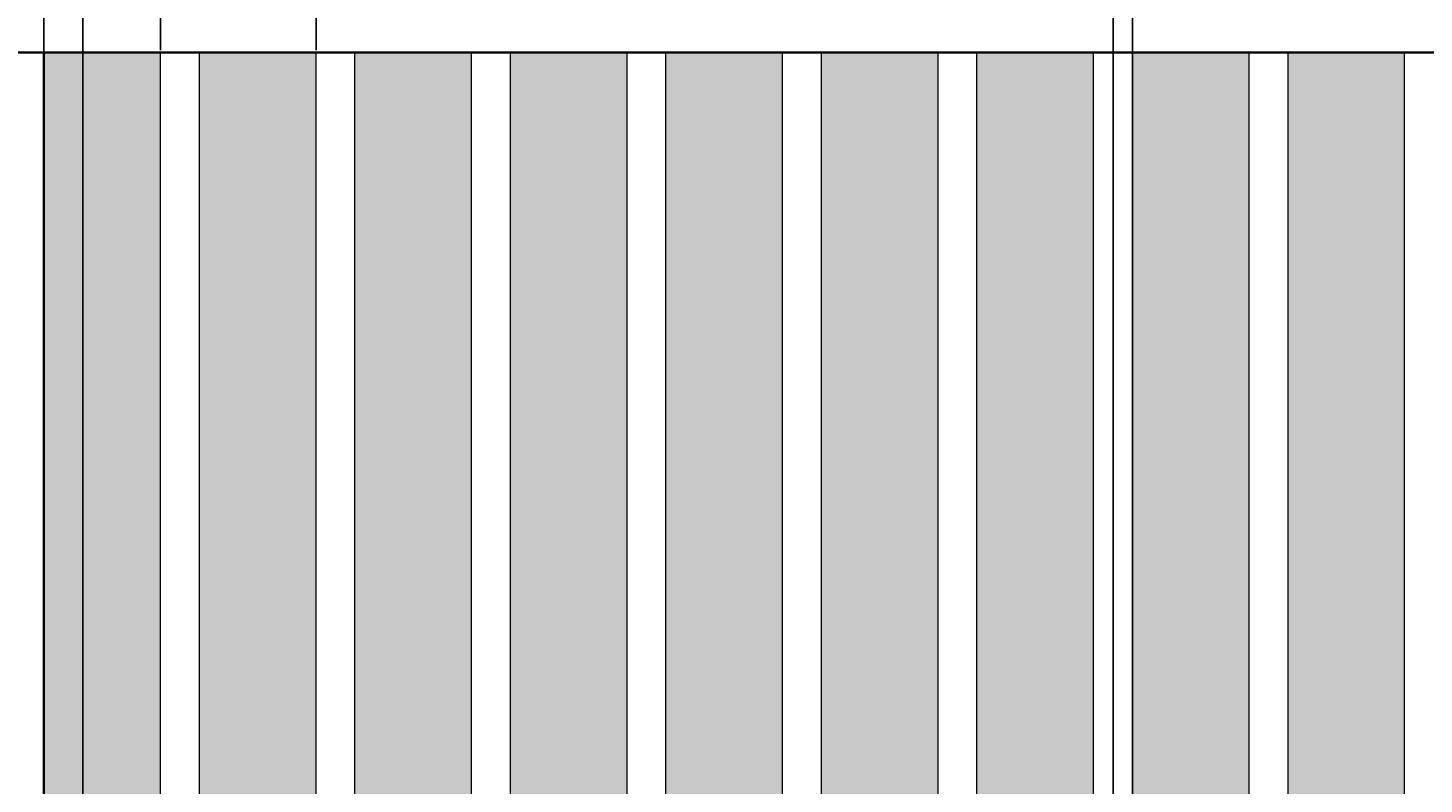
# Model space of a CAD drawing. Units: inches. Extents: x 4508 to 4723, y 847 to 1020.
# Tile 15 of 32: x 4550 to 4585, y 976 to 995. Entities that reach past the tile are written whole.
import ezdxf

# ---------------------------------------------------------------- set-up
doc = ezdxf.new("R2010")
doc.units = ezdxf.units.IN
for name, color, linetype, lineweight in [('A-ANNO-DIMS', 2, 'Continuous', 18), ('A-WALL', 7, 'Continuous', 35), ('A-WALL-FINS', 30, 'Continuous', 18), ('A-WALL-PATT', 254, 'Continuous', 13)]:
    doc.layers.add(name, color=color, linetype=linetype, lineweight=lineweight)
doc.styles.get("Standard").update_dxf_attribs({"font": 'arial.ttf'})
doc.dimstyles.get("Standard").update_dxf_attribs({"dimtxt": 0.18, "dimasz": 0.18, "dimexe": 0.18, "dimexo": 0.0625, "dimgap": 0.09, "dimtad": 0, "dimtih": 1, "dimtoh": 1, "dimdec": 4, "dimzin": 0, "dimdsep": 46, "dimtxsty": 'Standard', "dimcen": 0.09, "dimadec": 0, "dimazin": 0, "dimtfac": 1, "dimtdec": 4, "dimtofl": 0, "dimtmove": 0, "dimatfit": 3, "dimfxl": 1, "dimtolj": 1, "dimtzin": 0, "dimarcsym": 0})

# ---------------------------------------------------------------- blocks, each defined once
blk = doc.blocks.new('*D4')
at = {"layer": 'A-ANNO-DIMS', "color": 0, "lineweight": -2, "transparency": 16777216}
for p, q in [((4540.994, 994.809), (4540.994, 1002.877)), ((4541.174, 1002.697), (4545.345, 1002.697)), ((4549.814, 1002.697), (4545.643, 1002.697)), ((4549.994, 994.809), (4549.994, 1002.877))]:
    blk.add_line(p, q, dxfattribs=at)
at = {"layer": 'A-ANNO-DIMS', "color": 0, "lineweight": 9, "transparency": 16777216}
for points in [[(4541.174, 1002.727), (4541.174, 1002.667), (4540.994, 1002.697)], [(4549.814, 1002.727), (4549.814, 1002.667), (4549.994, 1002.697)]]:
    blk.add_solid(points, dxfattribs=at)
at = {"layer": 'Defpoints', "color": 0, "lineweight": 9, "transparency": 16777216}
for p in [(4549.994, 1002.697), (4540.994, 994.747), (4549.994, 994.747)]:
    blk.add_point(p, dxfattribs=at)
at = {"layer": 'A-ANNO-DIMS', "color": 0, "transparency": 16777216, "insert": (4545.494, 1002.697), "char_height": 0.18, "attachment_point": 5}
blk.add_mtext('\\A1;9', dxfattribs=at)
blk = doc.blocks.new('*D5')
at = {"layer": 'A-ANNO-DIMS', "color": 0, "lineweight": -2, "transparency": 16777216}
for p, q in [((4549.994, 994.809), (4549.994, 1002.877)), ((4550.174, 1002.697), (4551.345, 1002.697)), ((4552.814, 1002.697), (4551.643, 1002.697)), ((4552.994, 994.809), (4552.994, 1002.877))]:
    blk.add_line(p, q, dxfattribs=at)
at = {"layer": 'A-ANNO-DIMS', "color": 0, "lineweight": 9, "transparency": 16777216}
for points in [[(4550.174, 1002.727), (4550.174, 1002.667), (4549.994, 1002.697)], [(4552.814, 1002.727), (4552.814, 1002.667), (4552.994, 1002.697)]]:
    blk.add_solid(points, dxfattribs=at)
at = {"layer": 'Defpoints', "color": 0, "lineweight": 9, "transparency": 16777216}
for p in [(4552.994, 1002.697), (4549.994, 994.747), (4552.994, 994.747)]:
    blk.add_point(p, dxfattribs=at)
at = {"layer": 'A-ANNO-DIMS', "color": 0, "transparency": 16777216, "insert": (4551.494, 1002.697), "char_height": 0.18, "attachment_point": 5}
blk.add_mtext('\\A1;3', dxfattribs=at)
blk = doc.blocks.new('*D6')
at = {"layer": 'A-ANNO-DIMS', "color": 0, "lineweight": -2, "transparency": 16777216}
for p, q in [((4552.994, 994.809), (4552.994, 1002.877)), ((4553.174, 1002.697), (4554.842, 1002.697)), ((4556.814, 1002.697), (4555.146, 1002.697)), ((4556.994, 994.809), (4556.994, 1002.877))]:
    blk.add_line(p, q, dxfattribs=at)
at = {"layer": 'A-ANNO-DIMS', "color": 0, "lineweight": 9, "transparency": 16777216}
for points in [[(4553.174, 1002.727), (4553.174, 1002.667), (4552.994, 1002.697)], [(4556.814, 1002.727), (4556.814, 1002.667), (4556.994, 1002.697)]]:
    blk.add_solid(points, dxfattribs=at)
at = {"layer": 'Defpoints', "color": 0, "lineweight": 9, "transparency": 16777216}
for p in [(4556.994, 1002.697), (4552.994, 994.747), (4556.994, 994.747)]:
    blk.add_point(p, dxfattribs=at)
at = {"layer": 'A-ANNO-DIMS', "color": 0, "transparency": 16777216, "insert": (4554.994, 1002.697), "char_height": 0.18, "attachment_point": 5}
blk.add_mtext('\\A1;4', dxfattribs=at)
blk = doc.blocks.new('*D26')
at = {"layer": 'A-ANNO-DIMS', "color": 0, "lineweight": -2, "transparency": 16777216}
for p, q in [((4549.994, 904.809), (4549.994, 1002.877)), ((4550.174, 1002.697), (4550.371, 1002.697)), ((4550.814, 1002.697), (4550.617, 1002.697)), ((4550.994, 903.809), (4550.994, 1002.877))]:
    blk.add_line(p, q, dxfattribs=at)
at = {"layer": 'A-ANNO-DIMS', "color": 0, "lineweight": 9, "transparency": 16777216}
for points in [[(4550.174, 1002.727), (4550.174, 1002.667), (4549.994, 1002.697)], [(4550.814, 1002.727), (4550.814, 1002.667), (4550.994, 1002.697)]]:
    blk.add_solid(points, dxfattribs=at)
at = {"layer": 'Defpoints', "color": 0, "lineweight": 9, "transparency": 16777216}
for p in [(4550.994, 1002.697), (4549.994, 904.747), (4550.994, 903.747)]:
    blk.add_point(p, dxfattribs=at)
at = {"layer": 'A-ANNO-DIMS', "color": 0, "transparency": 16777216, "insert": (4550.494, 1002.697), "char_height": 0.18, "attachment_point": 5}
blk.add_mtext('\\A1;1', dxfattribs=at)
blk = doc.blocks.new('*D27')
at = {"layer": 'A-ANNO-DIMS', "color": 0, "lineweight": -2, "transparency": 16777216}
for p, q in [((4550.994, 903.809), (4550.994, 1002.877)), ((4551.174, 1002.697), (4563.918, 1002.697)), ((4577.314, 1002.697), (4564.57, 1002.697)), ((4577.494, 903.809), (4577.494, 1002.877))]:
    blk.add_line(p, q, dxfattribs=at)
at = {"layer": 'A-ANNO-DIMS', "color": 0, "lineweight": 9, "transparency": 16777216}
for points in [[(4551.174, 1002.727), (4551.174, 1002.667), (4550.994, 1002.697)], [(4577.314, 1002.727), (4577.314, 1002.667), (4577.494, 1002.697)]]:
    blk.add_solid(points, dxfattribs=at)
at = {"layer": 'Defpoints', "color": 0, "lineweight": 9, "transparency": 16777216}
for p in [(4577.494, 1002.697), (4550.994, 903.747), (4577.494, 903.747)]:
    blk.add_point(p, dxfattribs=at)
at = {"layer": 'A-ANNO-DIMS', "color": 0, "transparency": 16777216, "insert": (4564.244, 1002.697), "char_height": 0.18, "attachment_point": 5}
blk.add_mtext('\\A1;26.5', dxfattribs=at)
blk = doc.blocks.new('*D28')
at = {"layer": 'A-ANNO-DIMS', "color": 0, "lineweight": -2, "transparency": 16777216}
for p, q in [((4577.314, 1002.697), (4577.134, 1002.697)), ((4577.494, 903.809), (4577.494, 1002.877)), ((4577.994, 903.809), (4577.994, 1002.877)), ((4578.174, 1002.697), (4578.354, 1002.697))]:
    blk.add_line(p, q, dxfattribs=at)
at = {"layer": 'A-ANNO-DIMS', "color": 0, "lineweight": 9, "transparency": 16777216}
for points in [[(4577.314, 1002.727), (4577.314, 1002.667), (4577.494, 1002.697)], [(4578.174, 1002.727), (4578.174, 1002.667), (4577.994, 1002.697)]]:
    blk.add_solid(points, dxfattribs=at)
at = {"layer": 'Defpoints', "color": 0, "lineweight": 9, "transparency": 16777216}
for p in [(4577.994, 1002.697), (4577.494, 903.747), (4577.994, 903.747)]:
    blk.add_point(p, dxfattribs=at)
at = {"layer": 'A-ANNO-DIMS', "color": 0, "transparency": 16777216, "insert": (4578.608, 1002.697), "char_height": 0.18, "attachment_point": 5}
blk.add_mtext('\\A1;0.5', dxfattribs=at)
blk = doc.blocks.new('*D29')
at = {"layer": 'A-ANNO-DIMS', "color": 0, "lineweight": -2, "transparency": 16777216}
for p, q in [((4577.994, 903.809), (4577.994, 1002.877)), ((4578.174, 1002.697), (4590.773, 1002.697)), ((4603.814, 1002.697), (4591.214, 1002.697)), ((4603.994, 903.809), (4603.994, 1002.877))]:
    blk.add_line(p, q, dxfattribs=at)
at = {"layer": 'A-ANNO-DIMS', "color": 0, "lineweight": 9, "transparency": 16777216}
for points in [[(4578.174, 1002.727), (4578.174, 1002.667), (4577.994, 1002.697)], [(4603.814, 1002.727), (4603.814, 1002.667), (4603.994, 1002.697)]]:
    blk.add_solid(points, dxfattribs=at)
at = {"layer": 'Defpoints', "color": 0, "lineweight": 9, "transparency": 16777216}
for p in [(4603.994, 1002.697), (4577.994, 903.747), (4603.994, 903.747)]:
    blk.add_point(p, dxfattribs=at)
at = {"layer": 'A-ANNO-DIMS', "color": 0, "transparency": 16777216, "insert": (4590.994, 1002.697), "char_height": 0.18, "attachment_point": 5}
blk.add_mtext('\\A1;26', dxfattribs=at)

msp = doc.modelspace()

# ---------------------------------------------------------------- hatches: boundary and pattern name
at = {"layer": 'A-WALL-PATT', "transparency": 33554681}
h = msp.add_hatch(color=256, dxfattribs=at)
h.dxf.hatch_style = 1
h.paths.add_polyline_path([(4552.9938, 994.7469), (4549.9938, 994.7469), (4549.9938, 904.7469), (4552.9938, 904.7469)])
h.paths.add_polyline_path([(4556.9938, 994.7469), (4553.9938, 994.7469), (4553.9938, 904.7469), (4556.9938, 904.7469)])
h.paths.add_polyline_path([(4560.9938, 994.7469), (4557.9938, 994.7469), (4557.9938, 904.7469), (4560.9938, 904.7469)])
h.paths.add_polyline_path([(4564.9938, 994.7469), (4561.9938, 994.7469), (4561.9938, 904.7469), (4564.9938, 904.7469)])
h.paths.add_polyline_path([(4568.9938, 994.7469), (4565.9938, 994.7469), (4565.9938, 904.7469), (4568.9938, 904.7469)])
h.paths.add_polyline_path([(4572.9938, 994.7469), (4569.9938, 994.7469), (4569.9938, 904.7469), (4572.9938, 904.7469)])
h.paths.add_polyline_path([(4576.9938, 994.7469), (4573.9938, 994.7469), (4573.9938, 904.7469), (4576.9938, 904.7469)])
h.paths.add_polyline_path([(4580.9938, 994.7469), (4577.9938, 994.7469), (4577.9938, 904.7469), (4580.9938, 904.7469)])
h.paths.add_polyline_path([(4584.9938, 994.7469), (4581.9938, 994.7469), (4581.9938, 904.7469), (4584.9938, 904.7469)])

# ---------------------------------------------------------------- linework, layer by layer
at = {"layer": 'A-WALL'}
for p, q in [((4540.9938, 994.7469), (4693.9938, 994.7469)), ((4549.9938, 874.7469), (4549.9938, 994.7469))]:
    msp.add_line(p, q, dxfattribs=at)
at = {"layer": 'A-WALL-FINS'}
for p, q in [((4552.9938, 904.7469), (4552.9938, 994.7469)), ((4553.9938, 904.7469), (4553.9938, 994.7469)), ((4556.9938, 904.7469), (4556.9938, 994.7469)), ((4557.9938, 904.7469), (4557.9938, 994.7469)), ((4560.9938, 904.7469), (4560.9938, 994.7469)), ((4561.9938, 904.7469), (4561.9938, 994.7469)), ((4564.9938, 904.7469), (4564.9938, 994.7469)), ((4565.9938, 904.7469), (4565.9938, 994.7469)), ((4568.9938, 904.7469), (4568.9938, 994.7469)), ((4569.9938, 904.7469), (4569.9938, 994.7469)), ((4572.9938, 904.7469), (4572.9938, 994.7469)), ((4573.9938, 904.7469), (4573.9938, 994.7469)), ((4576.9938, 904.7469), (4576.9938, 994.7469)), ((4577.9938, 904.7469), (4577.9938, 994.7469)), ((4580.9938, 904.7469), (4580.9938, 994.7469)), ((4581.9938, 904.7469), (4581.9938, 994.7469)), ((4584.9938, 904.7469), (4584.9938, 994.7469))]:
    msp.add_line(p, q, dxfattribs=at)

# ---------------------------------------------------------------- dimensions: what is measured, and where the dimension line sits
at = {"layer": 'A-ANNO-DIMS'}
for base, p1, p2, override, picture, middle in [((4549.9938, 1002.6969), (4540.9938, 994.7469), (4549.9938, 994.7469), {"dimdec": 0, "dimlfac": 1, "dimrnd": 0, "dimzin": 0, "dimdsep": 46, "dimlunit": 2}, '*D4', (4545.4938, 1002.6969)), ((4552.9938, 1002.6969), (4549.9938, 994.7469), (4552.9938, 994.7469), {"dimdec": 0, "dimlfac": 1, "dimrnd": 0, "dimzin": 0, "dimdsep": 46, "dimlunit": 2}, '*D5', (4551.4938, 1002.6969)), ((4550.9938, 1002.6969), (4549.9938, 904.7469), (4550.9938, 903.7469), {"dimdec": 0, "dimlfac": 1, "dimrnd": 0, "dimzin": 0, "dimdsep": 46, "dimlunit": 2}, '*D26', (4550.4938, 1002.6969)), ((4577.4938, 1002.6969), (4550.9938, 903.7469), (4577.4938, 903.7469), {"dimdec": 1, "dimlfac": 1, "dimrnd": 0, "dimzin": 0, "dimdsep": 46, "dimlunit": 2}, '*D27', (4564.2438, 1002.6969)), ((4556.9938, 1002.6969), (4552.9938, 994.7469), (4556.9938, 994.7469), {"dimdec": 0, "dimlfac": 1, "dimrnd": 0, "dimzin": 0, "dimdsep": 46, "dimlunit": 2}, '*D6', (4554.9938, 1002.6969)), ((4577.9938, 1002.6969), (4577.4938, 903.7469), (4577.9938, 903.7469), {"dimdec": 1, "dimlfac": 1, "dimrnd": 0, "dimzin": 0, "dimdsep": 46, "dimlunit": 2}, '*D28', (4578.6083, 1002.6969)), ((4603.9938, 1002.6969), (4577.9938, 903.7469), (4603.9938, 903.7469), {"dimdec": 0, "dimlfac": 1, "dimrnd": 0, "dimzin": 0, "dimdsep": 46, "dimlunit": 2}, '*D29', (4590.9938, 1002.6969))]:
    dim = msp.add_linear_dim(base=base, p1=p1, p2=p2, dimstyle='Standard', override=override, dxfattribs=at)
    dim.commit()
    dim.dimension.update_dxf_attribs({"geometry": picture, "text_midpoint": middle})

doc.saveas('drawing.dxf')
